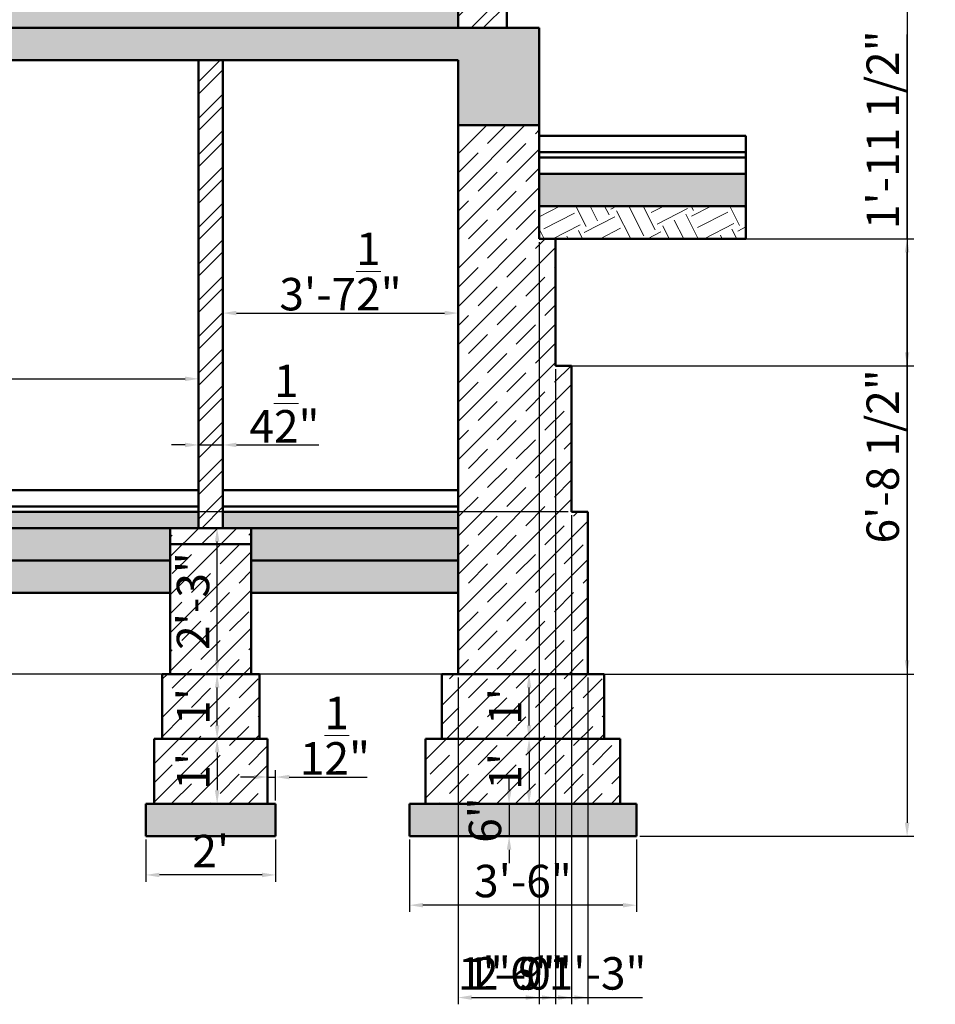
# Model space of a CAD drawing. Units: inches. Extents: x 1615 to 2231, y 1931 to 2519.
# Tile 4 of 6: x 2061 to 2231, y 1971 to 2153. Entities that reach past the tile are written whole.
import ezdxf

# ---------------------------------------------------------------- set-up
doc = ezdxf.new("R2010")
doc.units = ezdxf.units.IN
for name, color, linetype, lineweight in [('A-ANNO-DIMS', 2, 'Continuous', 18), ('A-SECT', 7, 'Continuous', 50), ('A-WALL-PATT', 8, 'Continuous', 13), ('C-TOPO-PATT', 252, 'Continuous', 13), ('S-FNDN', 1, 'Continuous', 50), ('S-FNDN-PATT', 8, 'Continuous', 13)]:
    doc.layers.add(name, color=color, linetype=linetype, lineweight=lineweight)
doc.styles.get("Standard").update_dxf_attribs({"font": 'arial.ttf'})
doc.dimstyles.new('ISO-25', dxfattribs={"dimtxt": 6, "dimasz": 2.5, "dimexe": 1.25, "dimexo": 0.625, "dimtad": 1, "dimdec": 1, "dimlunit": 4, "dimtxsty": 'Standard', "dimcen": 2.5, "dimadec": 0, "dimazin": 0, "dimtfac": 1, "dimtdec": 1, "dimtmove": 0, "dimatfit": 3, "dimfxl": 1, "dimarcsym": 0})

# ---------------------------------------------------------------- blocks, each defined once
blk = doc.blocks.new('*D27')
at = {"layer": 'A-ANNO-DIMS', "color": 0, "lineweight": -2, "transparency": 16777216}
for p, q in [((1974.87, 2077.27), (1974.87, 2087.86)), ((1977.37, 2086.61), (2091.87, 2086.61)), ((2094.37, 2077.27), (2094.37, 2087.86))]:
    blk.add_line(p, q, dxfattribs=at)
at = {"layer": 'A-ANNO-DIMS', "color": 0, "lineweight": 100, "transparency": 16777216}
for points in [[(1977.37, 2087.03), (1977.37, 2086.2), (1974.87, 2086.61)], [(2091.87, 2087.03), (2091.87, 2086.2), (2094.37, 2086.61)]]:
    blk.add_solid(points, dxfattribs=at)
at = {"layer": 'Defpoints', "color": 0, "lineweight": 100, "transparency": 16777216}
for p in [(2094.37, 2086.61), (1974.87, 2076.64), (2094.37, 2076.64)]:
    blk.add_point(p, dxfattribs=at)
at = {"layer": 'A-ANNO-DIMS', "color": 0, "transparency": 16777216, "insert": (2034.62, 2094.31), "char_height": 6, "attachment_point": 5}
blk.add_mtext('9\'-11{\\H1x;\\S1/2;}"', dxfattribs=at)
blk = doc.blocks.new('*D28')
at = {"layer": 'A-ANNO-DIMS', "color": 0, "lineweight": -2, "transparency": 16777216}
for p, q in [((2091.87, 2074.39), (2089.37, 2074.39)), ((2094.37, 2066.65), (2094.37, 2075.64)), ((2094.37, 2074.39), (2098.87, 2074.39)), ((2098.87, 2066.65), (2098.87, 2075.64)), ((2101.37, 2074.39), (2116.63, 2074.39))]:
    blk.add_line(p, q, dxfattribs=at)
at = {"layer": 'A-ANNO-DIMS', "color": 0, "lineweight": 100, "transparency": 16777216}
for points in [[(2091.87, 2074.81), (2091.87, 2073.97), (2094.37, 2074.39)], [(2101.37, 2074.81), (2101.37, 2073.97), (2098.87, 2074.39)]]:
    blk.add_solid(points, dxfattribs=at)
at = {"layer": 'Defpoints', "color": 0, "lineweight": 100, "transparency": 16777216}
for p in [(2098.87, 2074.39), (2094.37, 2066.03), (2098.87, 2066.03)]:
    blk.add_point(p, dxfattribs=at)
at = {"layer": 'A-ANNO-DIMS', "color": 0, "transparency": 16777216, "insert": (2110.25, 2082.04), "char_height": 6, "attachment_point": 5}
blk.add_mtext('4{\\H1x;\\S1/2;}"', dxfattribs=at)
blk = doc.blocks.new('*D29')
at = {"layer": 'A-ANNO-DIMS', "color": 0, "lineweight": -2, "transparency": 16777216}
for p, q in [((2098.87, 2092.67), (2098.87, 2100.02)), ((2142.37, 2092.67), (2142.37, 2100.02)), ((2101.37, 2098.77), (2139.87, 2098.77))]:
    blk.add_line(p, q, dxfattribs=at)
at = {"layer": 'A-ANNO-DIMS', "color": 0, "lineweight": 100, "transparency": 16777216}
for points in [[(2101.37, 2099.19), (2101.37, 2098.35), (2098.87, 2098.77)], [(2139.87, 2099.19), (2139.87, 2098.35), (2142.37, 2098.77)]]:
    blk.add_solid(points, dxfattribs=at)
at = {"layer": 'Defpoints', "color": 0, "lineweight": 100, "transparency": 16777216}
for p in [(2142.37, 2098.77), (2098.87, 2092.04), (2142.37, 2092.04)]:
    blk.add_point(p, dxfattribs=at)
at = {"layer": 'A-ANNO-DIMS', "color": 0, "transparency": 16777216, "insert": (2120.62, 2106.47), "char_height": 6, "attachment_point": 5}
blk.add_mtext('3\'-7{\\H1x;\\S1/2;}"', dxfattribs=at)
blk = doc.blocks.new('*D64')
at = {"layer": 'A-ANNO-DIMS', "color": 0, "lineweight": -2, "transparency": 16777216}
for p, q in [((2084.62, 2001.4), (2084.62, 1993.62)), ((2108.62, 2001.4), (2108.62, 1993.62)), ((2106.12, 1994.87), (2087.12, 1994.87))]:
    blk.add_line(p, q, dxfattribs=at)
at = {"layer": 'A-ANNO-DIMS', "color": 0, "lineweight": 100, "transparency": 16777216}
for points in [[(2087.12, 1995.29), (2087.12, 1994.46), (2084.62, 1994.87)], [(2106.12, 1995.29), (2106.12, 1994.46), (2108.62, 1994.87)]]:
    blk.add_solid(points, dxfattribs=at)
at = {"layer": 'Defpoints', "color": 0, "lineweight": 100, "transparency": 16777216}
for p in [(2084.62, 2002.03), (2108.62, 2002.03), (2084.62, 1994.87)]:
    blk.add_point(p, dxfattribs=at)
at = {"layer": 'A-ANNO-DIMS', "color": 0, "transparency": 16777216, "insert": (2096.62, 1998.51), "char_height": 6, "attachment_point": 5}
blk.add_mtext("2'", dxfattribs=at)
blk = doc.blocks.new('*D65')
at = {"layer": 'A-ANNO-DIMS', "color": 0, "lineweight": -2, "transparency": 16777216}
for p, q in [((2106.49, 2020.03), (2096.54, 2020.03)), ((2097.79, 2017.53), (2097.79, 2010.53)), ((2106.49, 2008.03), (2096.54, 2008.03))]:
    blk.add_line(p, q, dxfattribs=at)
at = {"layer": 'A-ANNO-DIMS', "color": 0, "lineweight": 100, "transparency": 16777216}
for points in [[(2097.38, 2017.53), (2098.21, 2017.53), (2097.79, 2020.03)], [(2097.38, 2010.53), (2098.21, 2010.53), (2097.79, 2008.03)]]:
    blk.add_solid(points, dxfattribs=at)
at = {"layer": 'Defpoints', "color": 0, "lineweight": 100, "transparency": 16777216}
for p in [(2107.12, 2020.03), (2097.79, 2008.03), (2107.12, 2008.03)]:
    blk.add_point(p, dxfattribs=at)
at = {"layer": 'A-ANNO-DIMS', "color": 0, "transparency": 16777216, "insert": (2094.16, 2014.03), "char_height": 6, "attachment_point": 5, "rotation": 90}
blk.add_mtext("1'", dxfattribs=at)
blk = doc.blocks.new('*D66')
at = {"layer": 'A-ANNO-DIMS', "color": 0, "lineweight": -2, "transparency": 16777216}
for p, q in [((2104.99, 2032.03), (2096.54, 2032.03)), ((2097.79, 2022.53), (2097.79, 2029.53)), ((2104.99, 2020.03), (2096.54, 2020.03))]:
    blk.add_line(p, q, dxfattribs=at)
at = {"layer": 'A-ANNO-DIMS', "color": 0, "lineweight": 100, "transparency": 16777216}
for points in [[(2097.38, 2029.53), (2098.21, 2029.53), (2097.79, 2032.03)], [(2097.38, 2022.53), (2098.21, 2022.53), (2097.79, 2020.03)]]:
    blk.add_solid(points, dxfattribs=at)
at = {"layer": 'Defpoints', "color": 0, "lineweight": 100, "transparency": 16777216}
for p in [(2097.79, 2032.03), (2105.62, 2032.03), (2105.62, 2020.03)]:
    blk.add_point(p, dxfattribs=at)
at = {"layer": 'A-ANNO-DIMS', "color": 0, "transparency": 16777216, "insert": (2094.16, 2026.03), "char_height": 6, "attachment_point": 5, "rotation": 90}
blk.add_mtext("1'", dxfattribs=at)
blk = doc.blocks.new('*D67')
at = {"layer": 'A-ANNO-DIMS', "color": 0, "lineweight": -2, "transparency": 16777216}
for p, q in [((2103.49, 2059.03), (2096.54, 2059.03)), ((2097.79, 2034.53), (2097.79, 2056.53)), ((2103.49, 2032.03), (2096.54, 2032.03))]:
    blk.add_line(p, q, dxfattribs=at)
at = {"layer": 'A-ANNO-DIMS', "color": 0, "lineweight": 100, "transparency": 16777216}
for points in [[(2097.38, 2056.53), (2098.21, 2056.53), (2097.79, 2059.03)], [(2097.38, 2034.53), (2098.21, 2034.53), (2097.79, 2032.03)]]:
    blk.add_solid(points, dxfattribs=at)
at = {"layer": 'Defpoints', "color": 0, "lineweight": 100, "transparency": 16777216}
for p in [(2097.79, 2059.03), (2104.12, 2059.03), (2104.12, 2032.03)]:
    blk.add_point(p, dxfattribs=at)
at = {"layer": 'A-ANNO-DIMS', "color": 0, "transparency": 16777216, "insert": (2094.1, 2045.53), "char_height": 6, "attachment_point": 5, "rotation": 90}
blk.add_mtext('2\'-3"', dxfattribs=at)
blk = doc.blocks.new('*D68')
at = {"layer": 'A-ANNO-DIMS', "color": 0, "lineweight": -2, "transparency": 16777216}
for p, q in [((2107.12, 2008.65), (2107.12, 2014.23)), ((2108.62, 2008.65), (2108.62, 2014.23)), ((2104.62, 2012.98), (2102.12, 2012.98)), ((2107.12, 2012.98), (2108.62, 2012.98)), ((2111.12, 2012.98), (2125.57, 2012.98))]:
    blk.add_line(p, q, dxfattribs=at)
at = {"layer": 'A-ANNO-DIMS', "color": 0, "lineweight": 100, "transparency": 16777216}
for points in [[(2104.62, 2013.39), (2104.62, 2012.56), (2107.12, 2012.98)], [(2111.12, 2013.39), (2111.12, 2012.56), (2108.62, 2012.98)]]:
    blk.add_solid(points, dxfattribs=at)
at = {"layer": 'Defpoints', "color": 0, "lineweight": 100, "transparency": 16777216}
for p in [(2108.62, 2012.98), (2107.12, 2008.03), (2108.62, 2008.03)]:
    blk.add_point(p, dxfattribs=at)
at = {"layer": 'A-ANNO-DIMS', "color": 0, "transparency": 16777216, "insert": (2119.59, 2020.63), "char_height": 6, "attachment_point": 5}
blk.add_mtext('1{\\H1x;\\S1/2;}"', dxfattribs=at)
blk = doc.blocks.new('*D69')
at = {"layer": 'A-ANNO-DIMS', "color": 0, "lineweight": -2, "transparency": 16777216}
for p, q in [((2133.37, 2001.4), (2133.37, 1988.03)), ((2175.37, 2001.4), (2175.37, 1988.03)), ((2172.87, 1989.28), (2135.87, 1989.28))]:
    blk.add_line(p, q, dxfattribs=at)
at = {"layer": 'A-ANNO-DIMS', "color": 0, "lineweight": 100, "transparency": 16777216}
for points in [[(2135.87, 1989.69), (2135.87, 1988.86), (2133.37, 1989.28)], [(2172.87, 1989.69), (2172.87, 1988.86), (2175.37, 1989.28)]]:
    blk.add_solid(points, dxfattribs=at)
at = {"layer": 'Defpoints', "color": 0, "lineweight": 100, "transparency": 16777216}
for p in [(2133.37, 2002.03), (2175.37, 2002.03), (2133.37, 1989.28)]:
    blk.add_point(p, dxfattribs=at)
at = {"layer": 'A-ANNO-DIMS', "color": 0, "transparency": 16777216, "insert": (2154.37, 1992.97), "char_height": 6, "attachment_point": 5}
blk.add_mtext('3\'-6"', dxfattribs=at)
blk = doc.blocks.new('*D70')
at = {"layer": 'A-ANNO-DIMS', "color": 0, "lineweight": -2, "transparency": 16777216}
for p, q in [((2171.74, 2020.03), (2154.25, 2020.03)), ((2155.5, 2017.53), (2155.5, 2010.53)), ((2171.74, 2008.03), (2154.25, 2008.03))]:
    blk.add_line(p, q, dxfattribs=at)
at = {"layer": 'A-ANNO-DIMS', "color": 0, "lineweight": 100, "transparency": 16777216}
for points in [[(2155.08, 2017.53), (2155.91, 2017.53), (2155.5, 2020.03)], [(2155.08, 2010.53), (2155.91, 2010.53), (2155.5, 2008.03)]]:
    blk.add_solid(points, dxfattribs=at)
at = {"layer": 'Defpoints', "color": 0, "lineweight": 100, "transparency": 16777216}
for p in [(2172.37, 2020.03), (2155.5, 2008.03), (2172.37, 2008.03)]:
    blk.add_point(p, dxfattribs=at)
at = {"layer": 'A-ANNO-DIMS', "color": 0, "transparency": 16777216, "insert": (2151.86, 2014.03), "char_height": 6, "attachment_point": 5, "rotation": 90}
blk.add_mtext("1'", dxfattribs=at)
blk = doc.blocks.new('*D71')
at = {"layer": 'A-ANNO-DIMS', "color": 0, "lineweight": -2, "transparency": 16777216}
for p, q in [((2168.74, 2032.03), (2154.25, 2032.03)), ((2155.5, 2022.53), (2155.5, 2029.53)), ((2168.74, 2020.03), (2154.25, 2020.03))]:
    blk.add_line(p, q, dxfattribs=at)
at = {"layer": 'A-ANNO-DIMS', "color": 0, "lineweight": 100, "transparency": 16777216}
for points in [[(2155.08, 2029.53), (2155.91, 2029.53), (2155.5, 2032.03)], [(2155.08, 2022.53), (2155.91, 2022.53), (2155.5, 2020.03)]]:
    blk.add_solid(points, dxfattribs=at)
at = {"layer": 'Defpoints', "color": 0, "lineweight": 100, "transparency": 16777216}
for p in [(2155.5, 2032.03), (2169.37, 2032.03), (2169.37, 2020.03)]:
    blk.add_point(p, dxfattribs=at)
at = {"layer": 'A-ANNO-DIMS', "color": 0, "transparency": 16777216, "insert": (2151.86, 2026.03), "char_height": 6, "attachment_point": 5, "rotation": 90}
blk.add_mtext("1'", dxfattribs=at)
blk = doc.blocks.new('*D72')
at = {"layer": 'A-ANNO-DIMS', "color": 0, "lineweight": -2, "transparency": 16777216}
for p, q in [((2151.81, 2010.53), (2151.81, 2013.03)), ((2174.74, 2008.03), (2150.56, 2008.03)), ((2151.81, 2008.03), (2151.81, 2002.03)), ((2174.74, 2002.03), (2150.56, 2002.03)), ((2151.81, 1999.53), (2151.81, 1997.03))]:
    blk.add_line(p, q, dxfattribs=at)
at = {"layer": 'A-ANNO-DIMS', "color": 0, "lineweight": 100, "transparency": 16777216}
for points in [[(2151.39, 2010.53), (2152.23, 2010.53), (2151.81, 2008.03)], [(2151.39, 1999.53), (2152.23, 1999.53), (2151.81, 2002.03)]]:
    blk.add_solid(points, dxfattribs=at)
at = {"layer": 'Defpoints', "color": 0, "lineweight": 100, "transparency": 16777216}
for p in [(2175.37, 2008.03), (2151.81, 2002.03), (2175.37, 2002.03)]:
    blk.add_point(p, dxfattribs=at)
at = {"layer": 'A-ANNO-DIMS', "color": 0, "transparency": 16777216, "insert": (2148.12, 2005.03), "char_height": 6, "attachment_point": 5, "rotation": 90}
blk.add_mtext('6"', dxfattribs=at)
blk = doc.blocks.new('*D79')
at = {"layer": 'A-ANNO-DIMS', "color": 0, "lineweight": -2, "transparency": 16777216}
for p, q in [((2151.99, 2476.53), (2226.69, 2476.53)), ((2225.44, 2474.03), (2225.44, 2004.53)), ((2175.99, 2002.03), (2226.69, 2002.03))]:
    blk.add_line(p, q, dxfattribs=at)
at = {"layer": 'A-ANNO-DIMS', "color": 0, "lineweight": 100, "transparency": 16777216}
for points in [[(2225.02, 2474.03), (2225.86, 2474.03), (2225.44, 2476.53)], [(2225.02, 2004.53), (2225.86, 2004.53), (2225.44, 2002.03)]]:
    blk.add_solid(points, dxfattribs=at)
at = {"layer": 'Defpoints', "color": 0, "lineweight": 100, "transparency": 16777216}
for p in [(2151.37, 2476.53), (2175.37, 2002.03), (2225.44, 2002.03)]:
    blk.add_point(p, dxfattribs=at)
at = {"layer": 'A-ANNO-DIMS', "color": 0, "transparency": 16777216, "insert": (2221.71, 2239.28), "char_height": 6, "attachment_point": 5, "rotation": 90}
blk.add_mtext('39\'-6 1/2"', dxfattribs=at)
blk = doc.blocks.new('*D84')
at = {"layer": 'A-ANNO-DIMS', "color": 0, "lineweight": -2, "transparency": 16777216}
for p, q in [((2157.37, 2111.9), (2157.37, 1970.95)), ((2142.37, 2031.4), (2142.37, 1970.95)), ((2144.87, 1972.2), (2154.87, 1972.2)), ((2157.37, 1972.2), (2176.5, 1972.2))]:
    blk.add_line(p, q, dxfattribs=at)
at = {"layer": 'A-ANNO-DIMS', "color": 0, "lineweight": 100, "transparency": 16777216}
for points in [[(2144.87, 1972.62), (2144.87, 1971.78), (2142.37, 1972.2)], [(2154.87, 1972.62), (2154.87, 1971.78), (2157.37, 1972.2)]]:
    blk.add_solid(points, dxfattribs=at)
at = {"layer": 'Defpoints', "color": 0, "lineweight": 100, "transparency": 16777216}
for p in [(2157.37, 2112.53), (2142.37, 2032.03), (2157.37, 1972.2)]:
    blk.add_point(p, dxfattribs=at)
at = {"layer": 'A-ANNO-DIMS', "color": 0, "transparency": 16777216, "insert": (2168.18, 1975.89), "char_height": 6, "attachment_point": 5}
blk.add_mtext('1\'-3"', dxfattribs=at)
blk = doc.blocks.new('*D85')
at = {"layer": 'A-ANNO-DIMS', "color": 0, "lineweight": -2, "transparency": 16777216}
for p, q in [((2160.37, 2088.4), (2160.37, 1970.95)), ((2142.37, 2031.4), (2142.37, 1970.95)), ((2144.87, 1972.2), (2157.87, 1972.2))]:
    blk.add_line(p, q, dxfattribs=at)
at = {"layer": 'A-ANNO-DIMS', "color": 0, "lineweight": 100, "transparency": 16777216}
for points in [[(2144.87, 1972.62), (2144.87, 1971.78), (2142.37, 1972.2)], [(2157.87, 1972.62), (2157.87, 1971.78), (2160.37, 1972.2)]]:
    blk.add_solid(points, dxfattribs=at)
at = {"layer": 'Defpoints', "color": 0, "lineweight": 100, "transparency": 16777216}
for p in [(2160.37, 2089.03), (2142.37, 2032.03), (2160.37, 1972.2)]:
    blk.add_point(p, dxfattribs=at)
at = {"layer": 'A-ANNO-DIMS', "color": 0, "transparency": 16777216, "insert": (2151.37, 1975.89), "char_height": 6, "attachment_point": 5}
blk.add_mtext('1\'-6"', dxfattribs=at)
blk = doc.blocks.new('*D86')
at = {"layer": 'A-ANNO-DIMS', "color": 0, "lineweight": -2, "transparency": 16777216}
for p, q in [((2163.37, 2061.4), (2163.37, 1970.95)), ((2142.37, 2031.4), (2142.37, 1970.95)), ((2144.87, 1972.2), (2160.87, 1972.2))]:
    blk.add_line(p, q, dxfattribs=at)
at = {"layer": 'A-ANNO-DIMS', "color": 0, "lineweight": 100, "transparency": 16777216}
for points in [[(2144.87, 1972.62), (2144.87, 1971.78), (2142.37, 1972.2)], [(2160.87, 1972.62), (2160.87, 1971.78), (2163.37, 1972.2)]]:
    blk.add_solid(points, dxfattribs=at)
at = {"layer": 'Defpoints', "color": 0, "lineweight": 100, "transparency": 16777216}
for p in [(2163.37, 2062.03), (2142.37, 2032.03), (2163.37, 1972.2)]:
    blk.add_point(p, dxfattribs=at)
at = {"layer": 'A-ANNO-DIMS', "color": 0, "transparency": 16777216, "insert": (2152.87, 1975.89), "char_height": 6, "attachment_point": 5}
blk.add_mtext('1\'-9"', dxfattribs=at)
blk = doc.blocks.new('*D87')
at = {"layer": 'A-ANNO-DIMS', "color": 0, "lineweight": -2, "transparency": 16777216}
for p, q in [((2142.37, 2031.4), (2142.37, 1970.95)), ((2166.37, 2031.4), (2166.37, 1970.95)), ((2144.87, 1972.2), (2163.87, 1972.2))]:
    blk.add_line(p, q, dxfattribs=at)
at = {"layer": 'A-ANNO-DIMS', "color": 0, "lineweight": 100, "transparency": 16777216}
for points in [[(2144.87, 1972.62), (2144.87, 1971.78), (2142.37, 1972.2)], [(2163.87, 1972.62), (2163.87, 1971.78), (2166.37, 1972.2)]]:
    blk.add_solid(points, dxfattribs=at)
at = {"layer": 'Defpoints', "color": 0, "lineweight": 100, "transparency": 16777216}
for p in [(2142.37, 2032.03), (2166.37, 2032.03), (2166.37, 1972.2)]:
    blk.add_point(p, dxfattribs=at)
at = {"layer": 'A-ANNO-DIMS', "color": 0, "transparency": 16777216, "insert": (2154.37, 1975.89), "char_height": 6, "attachment_point": 5}
blk.add_mtext('2\'-0"', dxfattribs=at)
blk = doc.blocks.new('*D88')
at = {"layer": 'A-ANNO-DIMS', "color": 0, "lineweight": -2, "transparency": 16777216}
for p, q in [((2162.74, 2062.03), (1621.79, 2062.03)), ((1623.04, 2059.53), (1623.04, 2034.53)), ((2165.74, 2032.03), (1621.79, 2032.03))]:
    blk.add_line(p, q, dxfattribs=at)
at = {"layer": 'A-ANNO-DIMS', "color": 0, "lineweight": 100, "transparency": 16777216}
for points in [[(1622.62, 2059.53), (1623.46, 2059.53), (1623.04, 2062.03)], [(1622.62, 2034.53), (1623.46, 2034.53), (1623.04, 2032.03)]]:
    blk.add_solid(points, dxfattribs=at)
at = {"layer": 'Defpoints', "color": 0, "lineweight": 100, "transparency": 16777216}
for p in [(2163.37, 2062.03), (1623.04, 2032.03), (2166.37, 2032.03)]:
    blk.add_point(p, dxfattribs=at)
at = {"layer": 'A-ANNO-DIMS', "color": 0, "transparency": 16777216, "insert": (1619.35, 2047.03), "char_height": 6, "attachment_point": 5, "rotation": 90}
blk.add_mtext('2\'-6"', dxfattribs=at)
blk = doc.blocks.new('*D89')
at = {"layer": 'A-ANNO-DIMS', "color": 0, "lineweight": -2, "transparency": 16777216}
for p, q in [((2157.99, 2112.53), (2226.69, 2112.53)), ((2225.44, 2034.53), (2225.44, 2110.03)), ((2166.99, 2032.03), (2226.69, 2032.03))]:
    blk.add_line(p, q, dxfattribs=at)
at = {"layer": 'A-ANNO-DIMS', "color": 0, "lineweight": 100, "transparency": 16777216}
for points in [[(2225.02, 2110.03), (2225.86, 2110.03), (2225.44, 2112.53)], [(2225.02, 2034.53), (2225.86, 2034.53), (2225.44, 2032.03)]]:
    blk.add_solid(points, dxfattribs=at)
at = {"layer": 'Defpoints', "color": 0, "lineweight": 100, "transparency": 16777216}
for p in [(2157.37, 2112.53), (2225.44, 2112.53), (2166.37, 2032.03)]:
    blk.add_point(p, dxfattribs=at)
at = {"layer": 'A-ANNO-DIMS', "color": 0, "transparency": 16777216, "insert": (2221.71, 2072.28), "char_height": 6, "attachment_point": 5, "rotation": 90}
blk.add_mtext('6\'-8 1/2"', dxfattribs=at)
blk = doc.blocks.new('*D90')
at = {"layer": 'A-ANNO-DIMS', "color": 0, "lineweight": -2, "transparency": 16777216}
for p, q in [((2225.44, 2112.53), (2225.44, 2150.3)), ((2157.99, 2112.53), (2226.69, 2112.53)), ((2225.44, 2091.53), (2225.44, 2110.03)), ((2160.99, 2089.03), (2226.69, 2089.03))]:
    blk.add_line(p, q, dxfattribs=at)
at = {"layer": 'A-ANNO-DIMS', "color": 0, "lineweight": 100, "transparency": 16777216}
for points in [[(2225.02, 2110.03), (2225.86, 2110.03), (2225.44, 2112.53)], [(2225.02, 2091.53), (2225.86, 2091.53), (2225.44, 2089.03)]]:
    blk.add_solid(points, dxfattribs=at)
at = {"layer": 'Defpoints', "color": 0, "lineweight": 100, "transparency": 16777216}
for p in [(2157.37, 2112.53), (2225.44, 2112.53), (2160.37, 2089.03)]:
    blk.add_point(p, dxfattribs=at)
at = {"layer": 'A-ANNO-DIMS', "color": 0, "transparency": 16777216, "insert": (2221.71, 2132.67), "char_height": 6, "attachment_point": 5, "rotation": 90}
blk.add_mtext('1\'-11 1/2"', dxfattribs=at)

msp = doc.modelspace()

# ---------------------------------------------------------------- hatches: boundary and pattern name
at = {"layer": 'A-WALL-PATT'}
h = msp.add_hatch(dxfattribs=at)
h.set_pattern_fill('ANSI32', color=256, scale=0.5)
h.paths.add_polyline_path([(1676.87, 2421.53), (1667.87, 2421.53), (1667.87, 2295.53), (1676.87, 2295.53)])
h.paths.add_polyline_path([(1676.87, 2277.53), (1667.87, 2277.53), (1667.87, 2151.53), (1676.87, 2151.53)])
h.paths.add_polyline_path([(1676.87, 2476.53), (1667.87, 2476.53), (1667.87, 2439.53), (1676.87, 2439.53)])
h.paths.add_polyline_path([(1894.37, 2421.29), (1889.87, 2421.29), (1889.87, 2295.53), (1894.37, 2295.53)])
h.paths.add_polyline_path([(1974.87, 2421.29), (1965.87, 2421.29), (1965.87, 2295.53), (1974.87, 2295.53)])
h.paths.add_polyline_path([(2151.37, 2421.29), (2142.37, 2421.29), (2142.37, 2295.53), (2151.37, 2295.53)])
h.paths.add_polyline_path([(2151.37, 2476.53), (2142.37, 2476.53), (2142.37, 2442.53), (2151.37, 2442.53)])
h.paths.add_polyline_path([(1974.87, 2277.53), (1965.87, 2277.53), (1965.87, 2151.53), (1974.87, 2151.53)])
h.paths.add_polyline_path([(1974.87, 2133.53), (1965.87, 2133.53), (1965.87, 2060.03), (1974.87, 2060.03)])
h.paths.add_polyline_path([(2098.87, 2145.53), (2094.37, 2145.53), (2094.37, 2059.03), (2098.87, 2059.03)])
h = msp.add_hatch(dxfattribs=at)
h.set_pattern_fill('DOTS', color=256, scale=0.5)
h.paths.add_polyline_path([(2142.37, 2442.53), (1839.37, 2442.53), (1676.87, 2442.53), (1676.87, 2439.53), (2142.37, 2439.53)])
h.paths.add_polyline_path([(1889.87, 2298.53), (1676.87, 2298.53), (1676.87, 2295.53), (1889.87, 2295.53)])
h.paths.add_polyline_path([(2142.37, 2298.53), (1974.87, 2298.53), (1974.87, 2295.53), (2142.37, 2295.53)])
h.paths.add_polyline_path([(1889.87, 2154.53), (1676.87, 2154.53), (1676.87, 2151.53), (1889.87, 2151.53)])
h.paths.add_polyline_path([(1965.87, 2154.53), (1894.37, 2154.53), (1894.37, 2151.53), (1965.87, 2151.53)])
h.paths.add_polyline_path([(2142.37, 2154.53), (1974.87, 2154.53), (1974.87, 2151.53), (2142.37, 2151.53)])
h.paths.add_polyline_path([(2094.37, 2062.03), (1974.87, 2062.03), (1974.87, 2059.03), (2094.37, 2059.03)])
h.paths.add_polyline_path([(2142.37, 2062.03), (2098.87, 2062.03), (2098.87, 2059.03), (2142.37, 2059.03)])
h.paths.add_polyline_path([(1956.87, 2049.53), (1693.37, 2049.53), (1693.37, 2046.53), (1956.87, 2046.53)])
h = msp.add_hatch(dxfattribs=at)
h.set_pattern_fill('AR-CONC', color=256, scale=0.1)
h.paths.add_polyline_path([(1898.87, 2151.53), (1667.87, 2151.53), (1667.87, 2145.53), (1679.87, 2145.53), (1682.87, 2145.53), (1889.87, 2145.53), (1889.87, 2133.53), (1974.87, 2133.53), (1974.87, 2145.53), (2142.37, 2145.53), (2142.37, 2133.53), (2157.37, 2133.53), (2157.37, 2151.53), (2155.87, 2151.53), (2151.37, 2151.53), (1965.87, 2151.53), (1965.87, 2139.53), (1898.87, 2139.53)])
h.paths.add_polyline_path([(1898.87, 2295.53), (1667.87, 2295.53), (1667.87, 2277.53), (1676.87, 2277.53), (1676.87, 2289.53), (1889.87, 2289.53), (1889.87, 2277.53), (1974.87, 2277.53), (1974.87, 2289.53), (2142.37, 2289.53), (2142.37, 2277.53), (2151.37, 2277.53), (2151.37, 2295.53), (1965.87, 2295.53), (1965.87, 2283.53), (1898.87, 2283.53)])
h.paths.add_polyline_path([(2142.37, 2439.53), (1676.87, 2439.53), (1667.87, 2439.53), (1667.87, 2421.53), (1676.87, 2421.53), (1676.87, 2433.53), (1889.87, 2433.53), (1889.87, 2421.29), (1898.87, 2421.29), (1898.87, 2433.53), (1965.87, 2433.53), (1965.87, 2421.29), (1974.87, 2421.29), (1974.87, 2433.53), (2142.37, 2433.53)])
h = msp.add_hatch(dxfattribs=at)
h.set_pattern_fill('ANSI32', color=256, scale=0.5)
h.paths.add_polyline_path([(2151.37, 2277.53), (2142.37, 2277.53), (2142.37, 2151.53), (2151.37, 2151.53)])
h.paths.add_polyline_path([(1894.37, 2277.53), (1889.87, 2277.53), (1889.87, 2151.53), (1894.37, 2151.53)])
h = msp.add_hatch(dxfattribs=at)
h.set_pattern_fill('JIS_STN_1E', color=256, scale=5)
h.paths.add_polyline_path([(1688.87, 2100.53), (1655.87, 2100.53), (1655.87, 2088.53), (1688.87, 2088.53)])
h.paths.add_polyline_path([(1685.87, 2112.53), (1658.87, 2112.53), (1658.87, 2100.53), (1685.87, 2100.53)])
h.paths.add_polyline_path([(1682.87, 2139.53), (1661.87, 2139.53), (1661.87, 2112.53), (1682.87, 2112.53)])
h.paths.add_polyline_path([(1688.87, 2088.53), (1655.87, 2088.53), (1652.87, 2088.53), (1652.87, 2082.53), (1688.87, 2082.53)])
h.paths.add_polyline_path([(1682.87, 2145.53), (1679.87, 2145.53), (1676.87, 2145.53), (1661.87, 2145.53), (1661.87, 2139.53), (1682.87, 2139.53)])
h.paths.add_polyline_path([(1974.87, 2057.03), (1956.87, 2057.03), (1956.87, 2044.03), (1974.87, 2044.03)])
h.paths.add_polyline_path([(1974.87, 2060.03), (1956.87, 2060.03), (1956.87, 2057.03), (1974.87, 2057.03)])
h.paths.add_polyline_path([(1980.87, 2032.03), (1950.87, 2032.03), (1950.87, 2020.03), (1980.87, 2020.03)])
h.paths.add_polyline_path([(1977.87, 2044.03), (1953.87, 2044.03), (1953.87, 2032.03), (1977.87, 2032.03)])
h.paths.add_polyline_path([(1983.87, 2020.03), (1947.87, 2020.03), (1947.87, 2008.03), (1983.87, 2008.03)])
h.paths.add_polyline_path([(2104.12, 2056.03), (2089.12, 2056.03), (2089.12, 2032.03), (2104.12, 2032.03)])
h.paths.add_polyline_path([(2104.12, 2059.03), (2089.12, 2059.03), (2089.12, 2056.03), (2104.12, 2056.03)])
h.paths.add_polyline_path([(2105.62, 2032.03), (2087.62, 2032.03), (2087.62, 2020.03), (2105.62, 2020.03)])
h.paths.add_polyline_path([(2107.12, 2020.03), (2086.12, 2020.03), (2086.12, 2008.03), (2107.12, 2008.03)])
h.paths.add_polyline_path([(2169.37, 2032.03), (2139.37, 2032.03), (2139.37, 2020.03), (2169.37, 2020.03)])
h.paths.add_polyline_path([(2172.37, 2020.03), (2136.37, 2020.03), (2136.37, 2008.03), (2172.37, 2008.03)])
h.paths.add_polyline_path([(2166.37, 2062.03), (2163.37, 2062.03), (2163.37, 2089.03), (2160.37, 2089.03), (2160.37, 2112.53), (2157.37, 2112.53), (2157.37, 2133.53), (2142.37, 2133.53), (2142.37, 2032.03), (2166.37, 2032.03)])
at = {"layer": 'C-TOPO-PATT'}
h = msp.add_hatch(dxfattribs=at)
h.set_pattern_fill('GRAVEL', color=256, scale=0.5, angle=27)
h.paths.add_polyline_path([(1956.87, 2046.53), (1693.37, 2046.53), (1693.37, 2040.53), (1953.87, 2040.53), (1953.87, 2044.03), (1956.87, 2044.03)])
h.paths.add_polyline_path([(2089.12, 2059.03), (1974.87, 2059.03), (1974.87, 2053.03), (2089.12, 2053.03)])
h.paths.add_polyline_path([(2142.37, 2059.03), (2104.12, 2059.03), (2104.12, 2053.03), (2142.37, 2053.03)])
h.paths.add_polyline_path([(2195.62, 2124.53), (2157.37, 2124.53), (2157.37, 2118.53), (2195.62, 2118.53)])
h = msp.add_hatch(dxfattribs=at)
h.set_pattern_fill('EARTH', color=256, angle=27)
h.paths.add_polyline_path([(2195.62, 2118.53), (2157.37, 2118.53), (2157.37, 2112.53), (2195.62, 2112.53)])
h = msp.add_hatch(dxfattribs=at)
h.set_pattern_fill('EARTH', color=256, angle=27)
h.paths.add_polyline_path([(1953.87, 2040.53), (1693.37, 2040.53), (1693.37, 2034.53), (1696.37, 2034.53), (1953.87, 2034.53)])
h.paths.add_polyline_path([(2089.12, 2053.03), (1974.87, 2053.03), (1974.87, 2047.03), (2089.12, 2047.03)])
h.paths.add_polyline_path([(2142.37, 2053.03), (2104.12, 2053.03), (2104.12, 2047.03), (2142.37, 2047.03)])
at = {"layer": 'S-FNDN-PATT'}
h = msp.add_hatch(dxfattribs=at)
h.set_pattern_fill('AR-CONC', color=256, scale=0.1)
h.paths.add_polyline_path([(1702.37, 2010.53), (1667.87, 2010.53), (1667.87, 2004.53), (1702.37, 2004.53)])
h.paths.add_polyline_path([(1986.87, 2008.03), (1944.87, 2008.03), (1944.87, 2002.03), (1986.87, 2002.03)])
h.paths.add_polyline_path([(2108.62, 2008.03), (2084.62, 2008.03), (2084.62, 2002.03), (2108.62, 2002.03)])
h.paths.add_polyline_path([(2175.37, 2008.03), (2133.37, 2008.03), (2133.37, 2002.03), (2175.37, 2002.03)])

# ---------------------------------------------------------------- linework, layer by layer
at = {"layer": 'A-SECT'}
for p, q in [((2151.37, 2476.53), (2151.37, 2151.53)), ((2142.37, 2289.53), (2142.37, 2151.53)), ((1667.87, 2151.53), (2151.37, 2151.53)), ((1974.87, 2145.53), (2142.37, 2145.53)), ((2094.37, 2145.53), (2094.37, 2059.03)), ((2098.87, 2145.53), (2098.87, 2059.03)), ((2142.37, 2145.53), (2142.37, 2032.03)), ((2142.37, 2133.53), (2157.37, 2133.53)), ((2157.37, 2128.53), (2195.62, 2128.53)), ((2157.37, 2127.53), (2195.62, 2127.53)), ((2157.37, 2124.53), (2195.62, 2124.53)), ((2157.37, 2118.53), (2195.62, 2118.53)), ((2157.37, 2112.53), (2195.62, 2112.53)), ((1974.87, 2063.03), (2094.37, 2063.03)), ((2098.87, 2063.03), (2142.37, 2063.03)), ((1974.87, 2062.03), (2094.37, 2062.03)), ((2098.87, 2062.03), (2142.37, 2062.03)), ((1974.87, 2059.03), (2142.37, 2059.03)), ((2089.12, 2056.03), (2104.12, 2056.03)), ((1974.87, 2053.03), (2089.12, 2053.03)), ((2104.12, 2053.03), (2142.37, 2053.03)), ((1974.87, 2047.03), (2089.12, 2047.03)), ((2104.12, 2047.03), (2142.37, 2047.03))]:
    msp.add_line(p, q, dxfattribs=at)
at = {"layer": 'S-FNDN'}
for p, q in [((2151.37, 2151.53), (2155.87, 2151.53)), ((2157.37, 2151.53), (2155.87, 2151.53)), ((2157.37, 2112.53), (2157.37, 2151.53)), ((2157.37, 2131.53), (2195.62, 2131.53)), ((2195.62, 2112.53), (2195.62, 2131.53)), ((2142.37, 2066.03), (2142.37, 2116.33)), ((2160.37, 2112.53), (2157.37, 2112.53)), ((2160.37, 2089.03), (2160.37, 2112.53)), ((2163.37, 2089.03), (2160.37, 2089.03)), ((2163.37, 2062.03), (2163.37, 2089.03)), ((1974.87, 2066.03), (2094.37, 2066.03)), ((2098.87, 2066.03), (2142.37, 2066.03)), ((2166.37, 2062.03), (2163.37, 2062.03)), ((2166.37, 2062.03), (2166.37, 2032.03)), ((2089.12, 2059.03), (2089.12, 2032.03)), ((2104.12, 2059.03), (2104.12, 2032.03)), ((2087.62, 2032.03), (2105.62, 2032.03)), ((2087.62, 2032.03), (2087.62, 2020.03)), ((2105.62, 2032.03), (2105.62, 2020.03)), ((2139.37, 2032.03), (2169.37, 2032.03)), ((2139.37, 2032.03), (2139.37, 2020.03)), ((2169.37, 2032.03), (2169.37, 2020.03)), ((2086.12, 2020.03), (2107.12, 2020.03)), ((2086.12, 2020.03), (2086.12, 2008.03)), ((2107.12, 2020.03), (2107.12, 2008.03)), ((2136.37, 2020.03), (2172.37, 2020.03)), ((2136.37, 2020.03), (2136.37, 2008.03)), ((2172.37, 2020.03), (2172.37, 2008.03)), ((2084.62, 2008.03), (2108.62, 2008.03)), ((2084.62, 2002.03), (2084.62, 2008.03)), ((2108.62, 2008.03), (2108.62, 2002.03)), ((2133.37, 2008.03), (2175.37, 2008.03)), ((2133.37, 2002.03), (2133.37, 2008.03)), ((2175.37, 2008.03), (2175.37, 2002.03)), ((2108.62, 2002.03), (2084.62, 2002.03)), ((2175.37, 2002.03), (2133.37, 2002.03))]:
    msp.add_line(p, q, dxfattribs=at)

# ---------------------------------------------------------------- dimensions: what is measured, and where the dimension line sits
at = {"layer": 'A-ANNO-DIMS'}
for base, p1, p2, override, picture, middle in [((2225.44, 2002.03), (2151.37, 2476.53), (2175.37, 2002.03), {"dimdec": 1, "dimlfac": 1, "dimrnd": 0, "dimzin": 1, "dimdsep": 46, "dimlunit": 4, "dimfrac": 2}, '*D79', (2221.71, 2239.28)), ((2225.44, 2112.53), (2160.37, 2089.03), (2157.37, 2112.53), {"dimdec": 1, "dimlfac": 1, "dimrnd": 0, "dimzin": 1, "dimdsep": 46, "dimlunit": 4, "dimfrac": 2}, '*D90', (2221.71, 2132.67)), ((2225.44, 2112.53), (2166.37, 2032.03), (2157.37, 2112.53), {"dimdec": 1, "dimlfac": 1, "dimrnd": 0, "dimzin": 1, "dimdsep": 46, "dimlunit": 4, "dimfrac": 2}, '*D89', (2221.71, 2072.28)), ((1623.04, 2032.03), (2163.37, 2062.03), (2166.37, 2032.03), {"dimdec": 1, "dimlfac": 1, "dimrnd": 0, "dimzin": 1, "dimdsep": 46, "dimlunit": 4, "dimfrac": 2}, '*D88', (1619.35, 2047.03)), ((2097.79, 2059.03), (2104.12, 2032.03), (2104.12, 2059.03), {"dimclrd": 0, "dimclre": 0, "dimclrt": 0}, '*D67', (2094.1, 2045.53)), ((2097.79, 2032.03), (2105.62, 2020.03), (2105.62, 2032.03), {"dimclrd": 0, "dimclre": 0, "dimclrt": 0}, '*D66', (2094.16, 2026.03)), ((2155.5, 2032.03), (2169.37, 2020.03), (2169.37, 2032.03), {"dimclrd": 0, "dimclre": 0, "dimclrt": 0}, '*D71', (2151.86, 2026.03)), ((2097.79, 2008.03), (2107.12, 2020.03), (2107.12, 2008.03), {"dimclrd": 0, "dimclre": 0, "dimclrt": 0}, '*D65', (2094.16, 2014.03)), ((2155.5, 2008.03), (2172.37, 2020.03), (2172.37, 2008.03), {"dimclrd": 0, "dimclre": 0, "dimclrt": 0}, '*D70', (2151.86, 2014.03))]:
    dim = msp.add_linear_dim(base=base, p1=p1, p2=p2, angle=90, dimstyle='ISO-25', override=override, dxfattribs=at)
    dim.commit()
    dim.dimension.update_dxf_attribs({"geometry": picture, "text_midpoint": middle})
for base, p1, p2, override, picture, middle in [((2142.37, 2098.77), (2098.87, 2092.04), (2142.37, 2092.04), {"dimclrd": 0, "dimclre": 0, "dimclrt": 0}, '*D29', (2120.62, 2106.47)), ((2157.37, 1972.2), (2142.37, 2032.03), (2157.37, 2112.53), {"dimdec": 1, "dimlfac": 1, "dimrnd": 0, "dimzin": 1, "dimdsep": 46, "dimlunit": 4, "dimfrac": 2}, '*D84', (2168.18, 1975.89)), ((2094.37, 2086.61), (1974.87, 2076.64), (2094.37, 2076.64), {"dimclrd": 0, "dimclre": 0, "dimclrt": 0}, '*D27', (2034.62, 2094.31)), ((2098.87, 2074.39), (2094.37, 2066.03), (2098.87, 2066.03), {"dimclrd": 0, "dimclre": 0, "dimclrt": 0}, '*D28', (2110.25, 2082.04)), ((2160.37, 1972.2), (2142.37, 2032.03), (2160.37, 2089.03), {"dimdec": 1, "dimlfac": 1, "dimrnd": 0, "dimzin": 1, "dimdsep": 46, "dimlunit": 4, "dimfrac": 2}, '*D85', (2151.37, 1975.89)), ((2163.37, 1972.2), (2142.37, 2032.03), (2163.37, 2062.03), {"dimdec": 1, "dimlfac": 1, "dimrnd": 0, "dimzin": 1, "dimdsep": 46, "dimlunit": 4, "dimfrac": 2}, '*D86', (2152.87, 1975.89)), ((2166.37, 1972.2), (2142.37, 2032.03), (2166.37, 2032.03), {"dimdec": 1, "dimlfac": 1, "dimrnd": 0, "dimzin": 1, "dimdsep": 46, "dimlunit": 4, "dimfrac": 2}, '*D87', (2154.37, 1975.89)), ((2108.62, 2012.98), (2107.12, 2008.03), (2108.62, 2008.03), {"dimclrd": 0, "dimclre": 0, "dimclrt": 0}, '*D68', (2119.59, 2020.63)), ((2084.62, 1994.87), (2108.62, 2002.03), (2084.62, 2002.03), {"dimclrd": 0, "dimclre": 0, "dimclrt": 0}, '*D64', (2096.62, 1998.51)), ((2133.37, 1989.28), (2175.37, 2002.03), (2133.37, 2002.03), {"dimclrd": 0, "dimclre": 0, "dimclrt": 0}, '*D69', (2154.37, 1992.97))]:
    dim = msp.add_linear_dim(base=base, p1=p1, p2=p2, dimstyle='ISO-25', override=override, dxfattribs=at)
    dim.commit()
    dim.dimension.update_dxf_attribs({"geometry": picture, "text_midpoint": middle})
dim = msp.add_linear_dim(base=(2151.81, 2002.03), p1=(2175.37, 2008.03), p2=(2175.37, 2002.03), angle=90, dimstyle='ISO-25', override={"dimclrd": 0, "dimclre": 0, "dimclrt": 0}, dxfattribs=at)
dim.commit()
dim.dimension.update_dxf_attribs({"geometry": '*D72', "text_midpoint": (2151.81, 2005.03), "dimtype": 160})

doc.saveas('drawing.dxf')
